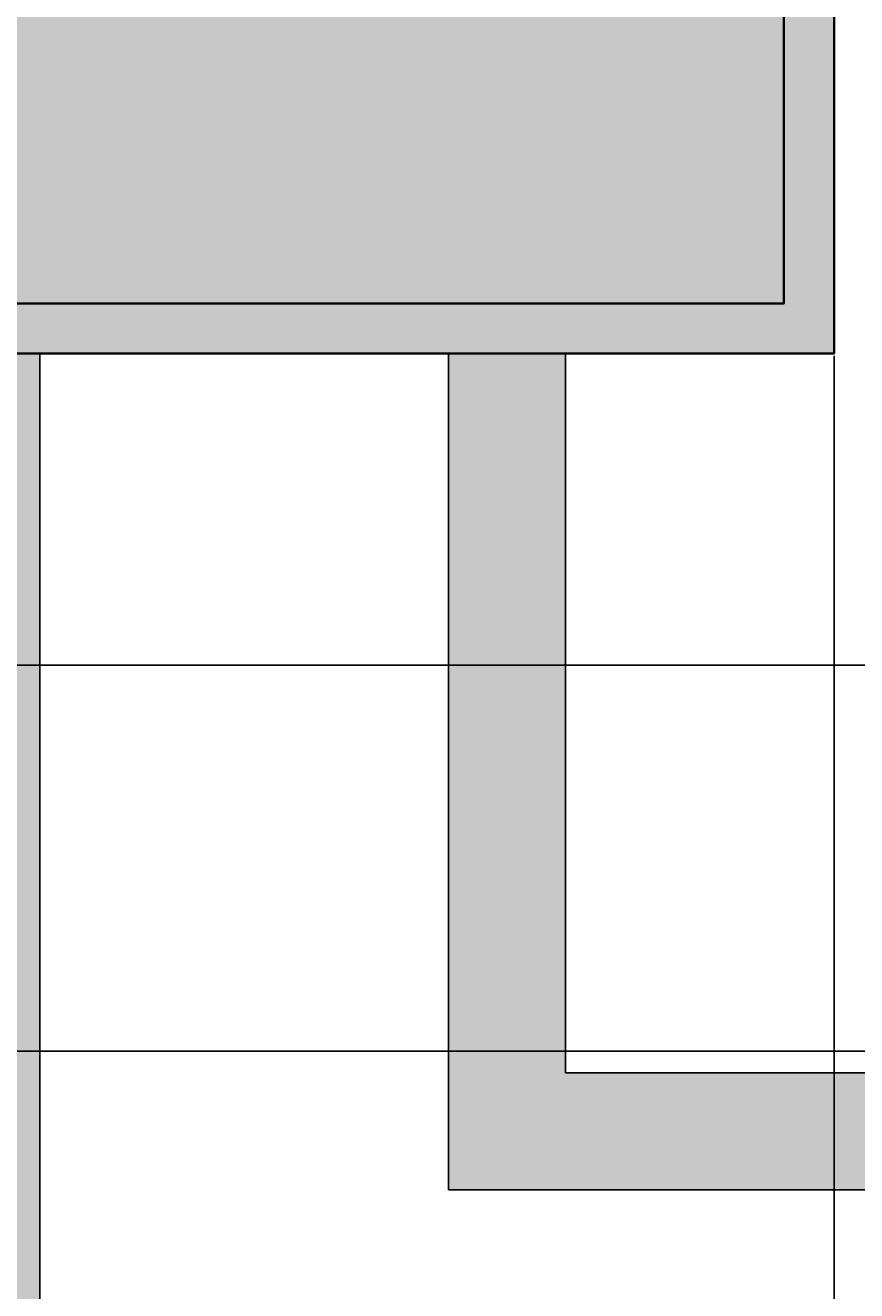
# Model space of a CAD drawing. Units: millimetres. Extents: x -11 to 280, y -4 to 208.
# Tile 12 of 55: x 42 to 67, y 126 to 164. Entities that reach past the tile are written whole.
import ezdxf

# ---------------------------------------------------------------- set-up
doc = ezdxf.new("R2010")
doc.units = ezdxf.units.MM
for name, color, linetype, lineweight in [('M-DIMS', 2, 'Continuous', 18), ('M-HYDR-EQPM', 7, 'Continuous', 35), ('M-HYDR-EQPM-PATT', 252, 'Continuous', 13), ('M-HYDR-SUCT', 7, 'Continuous', 25)]:
    doc.layers.add(name, color=color, linetype=linetype, lineweight=lineweight)
doc.layers.add('M-HYDR-SUCT-PATT', color=221, linetype='Continuous', lineweight=13, true_color=0xff7fdf)
doc.styles.get("Standard").update_dxf_attribs({"font": 'arial.ttf'})
doc.dimstyles.get("Standard").update_dxf_attribs({"dimtxt": 0.18, "dimasz": 0.18, "dimexe": 0.18, "dimexo": 0.0625, "dimgap": 0.09, "dimtad": 0, "dimtih": 1, "dimtoh": 1, "dimdec": 4, "dimzin": 0, "dimdsep": 46, "dimtxsty": 'Standard', "dimcen": 0.09, "dimadec": 0, "dimazin": 0, "dimtfac": 1, "dimtdec": 4, "dimtofl": 0, "dimtmove": 0, "dimatfit": 3, "dimfxl": 1, "dimtolj": 1, "dimtzin": 0, "dimarcsym": 0})

# ---------------------------------------------------------------- blocks, each defined once
blk = doc.blocks.new('*D5')
at = {"layer": 'Defpoints', "color": 0, "transparency": 16777216}
for p in [(24.759, 192.645), (-10.087, 11.435), (261.686, 11.435)]:
    blk.add_point(p, dxfattribs=at)
at = {"layer": 'M-DIMS', "color": 0, "lineweight": -2, "transparency": 16777216}
for p, q in [((24.696, 192.645), (-10.267, 192.645)), ((-10.087, 192.465), (-10.087, 102.222)), ((-10.087, 11.615), (-10.087, 101.858)), ((261.624, 11.435), (-10.267, 11.435))]:
    blk.add_line(p, q, dxfattribs=at)
at = {"layer": 'M-DIMS', "color": 0, "transparency": 16777216}
for points in [[(-10.117, 192.465), (-10.057, 192.465), (-10.087, 192.645)], [(-10.117, 11.615), (-10.057, 11.615), (-10.087, 11.435)]]:
    blk.add_solid(points, dxfattribs=at)
at = {"layer": 'M-DIMS', "color": 0, "transparency": 16777216, "insert": (-10.087, 102.04), "char_height": 0.18, "attachment_point": 5}
blk.add_mtext('\\A1;181.2', dxfattribs=at)
blk = doc.blocks.new('*D9')
at = {"layer": 'Defpoints', "color": 0, "transparency": 16777216}
for p in [(78.827, 207.495), (31.006, 98.021), (78.827, 98.149)]:
    blk.add_point(p, dxfattribs=at)
at = {"layer": 'M-DIMS', "color": 0, "lineweight": -2, "transparency": 16777216}
for p, q in [((31.006, 98.084), (31.006, 207.675)), ((31.186, 207.495), (54.52, 207.495)), ((78.647, 207.495), (55.313, 207.495)), ((78.827, 98.212), (78.827, 207.675))]:
    blk.add_line(p, q, dxfattribs=at)
at = {"layer": 'M-DIMS', "color": 0, "transparency": 16777216}
for points in [[(31.186, 207.525), (31.186, 207.465), (31.006, 207.495)], [(78.647, 207.525), (78.647, 207.465), (78.827, 207.495)]]:
    blk.add_solid(points, dxfattribs=at)
at = {"layer": 'M-DIMS', "color": 0, "transparency": 16777216, "insert": (54.917, 207.495), "char_height": 0.18, "attachment_point": 5}
blk.add_mtext('\\A1;47.82', dxfattribs=at)
blk = doc.blocks.new('*D14')
at = {"layer": 'Defpoints', "color": 0, "transparency": 16777216}
for p in [(-10.087, 144.661), (205.531, 144.661), (226.511, 133.123)]:
    blk.add_point(p, dxfattribs=at)
at = {"layer": 'M-DIMS', "color": 0, "lineweight": -2, "transparency": 16777216}
for p, q in [((205.469, 144.661), (-10.267, 144.661)), ((-10.087, 144.481), (-10.087, 139.074)), ((-10.087, 133.303), (-10.087, 138.71)), ((226.448, 133.123), (-10.267, 133.123))]:
    blk.add_line(p, q, dxfattribs=at)
at = {"layer": 'M-DIMS', "color": 0, "transparency": 16777216}
for points in [[(-10.117, 144.481), (-10.057, 144.481), (-10.087, 144.661)], [(-10.117, 133.303), (-10.057, 133.303), (-10.087, 133.123)]]:
    blk.add_solid(points, dxfattribs=at)
at = {"layer": 'M-DIMS', "color": 0, "transparency": 16777216, "insert": (-10.087, 138.892), "char_height": 0.18, "attachment_point": 5}
blk.add_mtext('\\A1;11.538', dxfattribs=at)
blk = doc.blocks.new('*D23')
at = {"layer": 'Defpoints', "color": 0, "transparency": 16777216}
for p in [(29.201, 153.977), (66.388, 153.977), (66.388, -3.415)]:
    blk.add_point(p, dxfattribs=at)
at = {"layer": 'M-DIMS', "color": 0, "lineweight": -2, "transparency": 16777216}
for p, q in [((29.201, 153.914), (29.201, -3.595)), ((66.388, 153.914), (66.388, -3.595)), ((29.381, -3.415), (47.331, -3.415)), ((66.208, -3.415), (48.258, -3.415))]:
    blk.add_line(p, q, dxfattribs=at)
at = {"layer": 'M-DIMS', "color": 0, "transparency": 16777216}
for points in [[(29.381, -3.385), (29.381, -3.445), (29.201, -3.415)], [(66.208, -3.385), (66.208, -3.445), (66.388, -3.415)]]:
    blk.add_solid(points, dxfattribs=at)
at = {"layer": 'M-DIMS', "color": 0, "transparency": 16777216, "insert": (47.795, -3.415), "char_height": 0.18, "attachment_point": 5}
blk.add_mtext('\\A1;37.186', dxfattribs=at)

msp = doc.modelspace()

# ---------------------------------------------------------------- hatches: boundary and pattern name
at = {"layer": 'M-HYDR-EQPM-PATT'}
h = msp.add_hatch(color=256, dxfattribs=at)
h.set_gradient(color1=(153, 153, 0), color2=(255, 255, 0), tint=1, name='INVCYLINDER')
h.paths.add_polyline_path([(64.8875, 177.7412), (30.7015, 177.7412), (30.7015, 155.4768), (64.8875, 155.4768)])
h.paths.add_polyline_path([(52.0736, 184.1929), (52.0736, 192.645), (24.7588, 192.645), (24.7588, 184.1929), (34.0713, 184.1929), (34.0713, 179.2412), (35.5061, 179.2412), (35.5061, 185.6276), (26.1935, 185.6276), (26.1935, 191.2103), (50.6389, 191.2103), (50.6389, 185.6276), (41.792, 185.6276), (41.792, 179.2412), (43.2268, 179.2412), (43.2268, 184.1929)])
h = msp.add_hatch(color=256, dxfattribs=at)
h.set_gradient(color1=(153, 153, 0), color2=(153, 153, 0), tint=1, name='INVCYLINDER')
h.paths.add_polyline_path([(26.1935, 191.2103), (26.1935, 185.6276), (35.5061, 185.6276), (35.5061, 179.2412), (41.792, 179.2412), (41.792, 185.6276), (50.6389, 185.6276), (50.6389, 191.2103)])
h.paths.add_polyline_path([(29.2015, 153.9768), (66.3875, 153.9768), (66.3875, 179.2412), (29.2015, 179.2412)])
h.paths.add_polyline_path([(30.7015, 177.7412), (64.8875, 177.7412), (64.8875, 155.4768), (30.7015, 155.4768)], flags=16)
at = {"layer": 'M-HYDR-SUCT-PATT'}
h = msp.add_hatch(color=256, dxfattribs=at)
h.set_gradient(color1=(255, 127, 223), color2=(255, 127, 223), tint=1, name='INVCYLINDER')
h.paths.add_polyline_path([(91.3629, 155.4768), (91.3629, 132.4768), (58.3629, 132.4768), (58.3629, 153.9768), (54.8629, 153.9768), (54.8629, 128.9768), (94.8629, 128.9768), (94.8629, 151.9768), (205.5315, 151.9768), (205.5315, 155.4768)])
h.paths.add_polyline_path([(91.3, 114.9452, 1), (78.8273, 114.9452), (78.8273, 108.8141), (42.6453, 108.8141), (42.6453, 153.9768), (39.1453, 153.9768), (39.1453, 105.3141), (78.8273, 105.3141), (78.8273, 98.1491, 1), (91.3, 98.1491), (91.3, 105.3141), (95.5776, 105.3141), (95.5776, 108.8141), (91.3, 108.8141)])
h.paths.add_polyline_path([(228.7, 138.4081), (232.2, 138.4081), (232.2, 144.6609), (228.7, 144.6609)])
h.paths.add_polyline_path([(253.1005, 151.9768, 1), (253.1005, 155.4768), (252.6001, 155.4768), (253.5249, 153.991, -0.1401047), (253.6005, 153.7268, -0.7542249), (252.676, 153.4626), (251.4221, 155.4768), (236.9353, 155.4768), (236.9353, 151.9768)])
h.paths.add_polyline_path([(30.8182, 40.7626), (30.8182, 36.7626), (60.8182, 36.7626), (60.8182, 40.7626)])

# ---------------------------------------------------------------- linework, layer by layer
at = {"layer": 'M-HYDR-EQPM'}
for points in [[(29.2015, 179.2412), (66.3875, 179.2412), (66.3875, 153.9768), (29.2015, 153.9768)], [(30.7015, 177.7412), (64.8875, 177.7412), (64.8875, 155.4768), (30.7015, 155.4768)]]:
    msp.add_lwpolyline(points, close=True, dxfattribs=at)
at = {"layer": 'M-HYDR-SUCT'}
for points in [[(58.3629, 153.9768), (58.3629, 132.4768), (91.3629, 132.4768), (91.3629, 155.4768), (205.5315, 155.4768)], [(78.8273, 108.8141), (42.6453, 108.8141), (42.6453, 153.9768)], [(54.8629, 153.9768), (54.8629, 128.9768), (94.8629, 128.9768), (94.8629, 151.9768), (205.5315, 151.9768)]]:
    msp.add_lwpolyline(points, dxfattribs=at)

# ---------------------------------------------------------------- dimensions: what is measured, and where the dimension line sits
at = {"layer": 'M-DIMS'}
for base, p1, p2, override, picture, middle in [((78.8273, 207.495), (31.0059, 98.0213), (78.8273, 98.1491), {"dimdec": 2, "dimlfac": 1, "dimrnd": 0, "dimzin": 0, "dimdsep": 46, "dimlunit": 2}, '*D9', (54.9166, 207.495)), ((66.3875, -3.4154), (29.2015, 153.9768), (66.3875, 153.9768), {"dimdec": 3, "dimlfac": 1, "dimrnd": 0, "dimzin": 0, "dimdsep": 46, "dimlunit": 2}, '*D23', (47.7945, -3.4154))]:
    dim = msp.add_linear_dim(base=base, p1=p1, p2=p2, dimstyle='Standard', override=override, dxfattribs=at)
    dim.commit()
    dim.dimension.update_dxf_attribs({"geometry": picture, "text_midpoint": middle})
for base, p1, p2, override, picture, middle in [((-10.0865, 11.4346), (24.7588, 192.645), (261.6863, 11.4346), {"dimdec": 1, "dimlfac": 1, "dimrnd": 0, "dimzin": 0, "dimdsep": 46, "dimlunit": 2}, '*D5', (-10.0865, 102.0398)), ((-10.0865, 144.6609), (226.5106, 133.1228), (205.5315, 144.6609), {"dimdec": 3, "dimlfac": 1, "dimrnd": 0, "dimzin": 0, "dimdsep": 46, "dimlunit": 2}, '*D14', (-10.0865, 138.8918))]:
    dim = msp.add_linear_dim(base=base, p1=p1, p2=p2, angle=90, dimstyle='Standard', override=override, dxfattribs=at)
    dim.commit()
    dim.dimension.update_dxf_attribs({"geometry": picture, "text_midpoint": middle})

doc.saveas('drawing.dxf')
